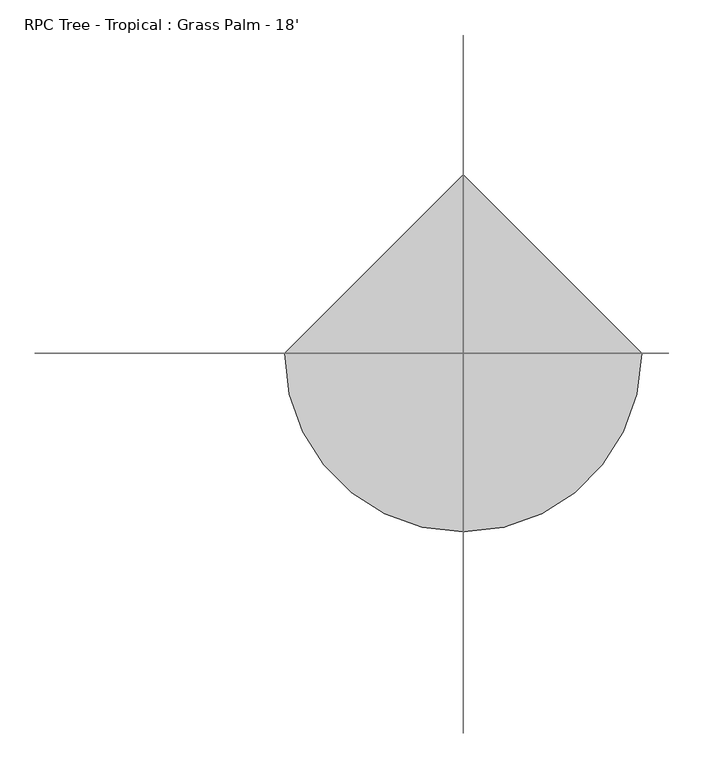
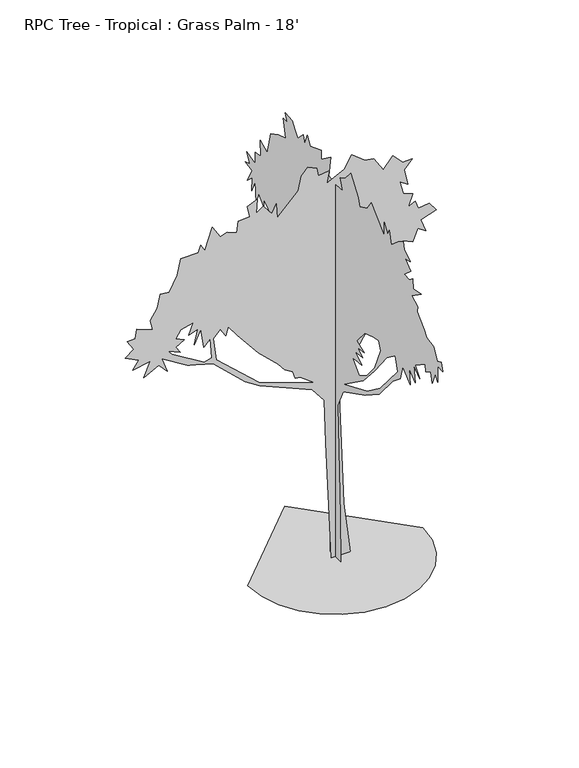
"""IFC4 building model written with IfcOpenShell, lengths in millimetres: geographic element geometry, RPC Tree - Tropical : Grass Palm - 18'."""

from ifc_helpers import new_model, si_unit, origin, place, context, project, spatial, triangles, source, transform, mapped, element, save


def rpc_tree_tropical_grass_palm_18_ffc4a38a(model_context):
    return source(origin(), model_context, "Body", "Tessellation", [
        triangles([(197.8251161, -0.0004657, 0.0001367), (109.1148514, -0.0002635, 694.5605118), (43.5490633, 0.0002048, 2380.5060047), (409.1686295, 0.0003079, 2962.5546341), (570.4154732, 0.000405, 3409.2137077), (607.6747178, 0.0004576, 3623.4372597), (719.4525244, 0.0004509, 3660.6992294), (654.2481468, 0.0004936, 3781.8063721), (747.397621, 0.0005252, 3949.4717194), (775.3401741, 0.0005007, 3874.9480705), (877.80376, 0.0005308, 4042.6134178), (1008.2098989, 0.0004934, 3977.4115837), (1073.4142765, 0.0005291, 4145.0772217), (1175.8753189, 0.0004934, 4070.5535728), (1110.6734848, 0.0005514, 4247.5407349), (1315.5981857, 0.0005381, 4312.742569), (1222.4487843, 0.0005851, 4433.8244225), (1082.7284609, 0.0006012, 4415.2060822), (1039.2334414, 0.0006388, 4529.6586891), (952.3222492, 0.0006386, 4480.4079163), (1008.2098989, 0.0006732, 4638.7514488), (886.9528381, 0.0007051, 4688.7640938), (840.544479, 0.0007593, 4862.3223953), (943.0055214, 0.0007261, 4797.0952721), (896.4321287, 0.0007914, 5011.3441132), (998.8957146, 0.0008063, 5123.1297318), (877.80376, 0.0008246, 5123.1297318), (747.397621, 0.0008797, 5253.5334), (626.3056664, 0.0008575, 5104.4861023), (503.8725509, 0.0009294, 5301.1072403), (384.1216845, 0.0009523, 5318.7352341), (216.4545022, 0.0010156, 5458.4604263), (113.9921609, 0.0009855, 5290.795079), (-109.5623986, 0.0009889, 5179.0094604), (-81.6183375, 0.0010277, 5337.3532837), (-221.3396873, 0.0010437, 5318.7352341), (-239.9693097, 0.0010769, 5430.5202713), (-361.0610281, 0.0011104, 5486.4005814), (-444.8937381, 0.0010978, 5393.2585922), (-482.1529827, 0.0010527, 5206.9496155), (-752.2819885, 0.0010175, 4927.5242294), (-770.9103573, 0.0010735, 5123.1297318), (-826.8005505, 0.0010516, 5011.3441132), (-938.5783207, 0.0011065, 5151.0698868), (-1031.7252514, 0.0011028, 5085.8680527), (-1013.0943392, 0.0011506, 5272.1514496), (-1143.5030216, 0.0011551, 5216.2711395), (-1115.557925, 0.0011104, 5067.2244232), (-1264.5950489, 0.0011304, 5057.9278976), (-1283.2232723, 0.0010926, 4908.8806), (-1404.3152996, 0.0011236, 4955.4643845), (-1497.4622303, 0.0011301, 4927.5242294), (-1599.9257435, 0.0011911, 5095.1895767), (-1702.389402, 0.0011281, 4806.4170868), (-1748.9628674, 0.0011604, 4899.5590759), (-1786.2220757, 0.0011407, 4806.4170868), (-2009.7751453, 0.0011745, 4806.4170868), (-2056.3486107, 0.0011233, 4592.1932442), (-2158.8122692, 0.0010856, 4396.5624527), (-2279.9041512, 0.0011064, 4405.8842674), (-2317.1635048, 0.0010639, 4228.8971054), (-2410.3102901, 0.00104, 4089.1972023), (-2377.0008408, 0.0009991, 3957.4473953), (-2587.2949814, 0.0010515, 4033.2916031), (-2605.9133217, 0.0010214, 3912.2100403), (-2708.3768349, 0.0010343, 3902.8882256), (-2624.5569511, 0.0009862, 3772.4845573), (-2736.3166992, 0.0009803, 3688.6390938), (-2559.355117, 0.0009282, 3595.4973953), (-2633.853186, 0.0009091, 3483.7117767), (-2410.3102901, 0.000888, 3530.2955612), (-2494.1431091, 0.0008475, 3334.6900589), (-2298.535136, 0.0008458, 3437.1535721), (-2186.7573658, 0.000796, 3316.0464294), (-2261.2733116, 0.0008604, 3511.6772209), (-1928.0074619, 0.0007539, 3305.1500015), (-1586.5374619, 0.000677, 3211.8556961), (-1169.4034029, 0.0005069, 2817.7745178), (-980.3029541, 0.0004448, 2694.5084953), (-299.9587802, 0.0002625, 2401.7378483), (-143.374379, 0.000185, 2203.9150394), (-126.1084725, 2.08e-05, 1609.6107628), (-53.6737587, -0.0004278, 0.0001367), (-1497.4622303, 0.0008957, 3651.4027039), (-1422.9462845, 0.000854, 3539.6173759), (-1395.0011879, 0.0008802, 3651.4027039), (-1273.9091606, 0.0008189, 3493.0335915), (-1002.0681953, 0.0003602, 3156.4073364), (-744.7432772, 0.0005791, 2905.2014488), (-659.9860233, 0.000538, 2801.1377426), (-556.6715083, 0.0005054, 2738.5520279), (-519.4122637, 0.0004719, 2636.0885147), (-454.2079225, 0.0004596, 2626.7667), (-267.9141337, 0.0003934, 2487.0438332), (-995.0831566, 0.0005747, 2749.8295372), (-1549.5677708, 0.0007954, 3253.765638), (-1590.6116318, 0.0008844, 3558.2354256), (-2019.0918732, 0.0008854, 3520.9737465), (-2074.9794502, 0.0009166, 3604.8192101), (-1963.20168, 0.0009175, 3670.0207535), (-2074.9794502, 0.0009495, 3725.9007729), (-2009.7751453, 0.0009676, 3828.3645767), (-1851.4239098, 0.0009538, 3865.6262558), (-1907.3141029, 0.0009217, 3716.604538), (-1791.7262455, 0.0009145, 3754.1964294), (-1838.0305412, 0.0008682, 3558.4641907), (-1748.9628674, 0.0009054, 3744.5444023), (-1711.7036591, 0.0008288, 3483.7117767), (-1627.8708401, 0.000839, 3567.5572403), (-1608.65835, 0.0007633, 3299.7651558), (-1708.7927902, 0.0007706, 3271.2916031), (-2130.8671726, 0.0009048, 3530.2955612), (-2177.4431087, 0.000927, 3586.1755806), (0.0001009, -125.9822357, 0.0001592), (6.27e-05, -114.0061317, 632.7801258), (3.21e-05, -52.0852428, 2115.3046051), (1.35e-05, -175.1038104, 2373.6836014), (-6.14e-05, -671.5328476, 2630.4243256), (-0.0001496, -990.5162842, 2836.0117767), (-0.0001562, -1298.9586491, 3200.2479744), (-0.0001816, -1467.3098557, 3334.6900589), (-0.00019, -1523.1974327, 3539.6173759), (-0.0002153, -1690.8629253, 3390.5700783), (-0.0002111, -1662.9202995, 3595.4973953), (-0.0002322, -1802.6406956, 3483.7373566), (-0.0002266, -1765.3814873, 3707.2827232), (-0.0002477, -1905.101738, 3604.8192101), (-0.0002322, -1802.6406956, 3725.9007729), (-0.000266, -2026.196236, 3874.9480705), (-0.0002688, -2044.8246048, 3781.8063721), (-0.0002843, -2147.2882633, 3837.6863914), (-0.0002899, -2184.5450008, 3707.2827232), (-0.0002997, -2249.7493057, 3874.9480705), (-0.0003096, -2314.9536106, 3800.4244217), (-0.0003096, -2314.9536106, 4023.9697884), (-0.0003265, -2426.7289101, 4014.6735535), (-0.0003208, -2389.4721725, 4126.4335922), (-0.0003068, -2296.3227711, 4079.8753876), (-0.0002955, -2221.8042091, 4238.2189201), (-0.0002716, -2063.4555897, 4266.1590752), (-0.0002632, -2007.5653965, 4340.6824333), (-0.0002792, -1849.2141609, 4489.729731), (-0.0002806, -1858.5282726, 4564.2280907), (-0.0002609, -1728.1221336, 4638.7514488), (-0.0002933, -1942.3609463, 4787.7987465), (-0.0002652, -1756.0672302, 4750.5370674), (-0.0002638, -1746.7531185, 4880.9404449), (-0.0002525, -1672.2345566, 4825.0607162), (-0.0002356, -1560.4567863, 4834.3569511), (-0.0002567, -1700.177037, 4955.4643845), (-0.0002384, -1579.0876259, 5057.9278976), (-0.0002553, -1690.8629253, 5085.8680527), (-0.0002342, -1551.1425293, 5169.6879364), (-0.0002314, -1532.5116898, 5262.854924), (-0.0002145, -1420.7339195, 5197.6530899), (-0.0001906, -1262.3826839, 5057.9278976), (-0.0001836, -1215.8092186, 5225.5932449), (-0.000178, -1178.5499376, 5151.0698868), (-0.0002067, -1104.0339191, 5272.1514496), (-0.0001667, -1104.0339191, 5085.8680527), (-0.0001811, -934.8191025, 5242.9666031), (-0.0001617, -805.9598167, 5355.9969131), (-0.0001497, -726.4933737, 5236.9472031), (-0.0001237, -554.4617231, 5151.0698868), (-0.0001181, -517.2024785, 5253.5334), (-9.28e-05, -349.5370585, 5486.4005814), (-7.45e-05, -228.4440684, 5346.6748077), (-5.62e-05, -107.3520956, 5281.4729736), (-6.46e-05, -163.2409807, 5132.4512558), (-4.21e-05, -14.2045188, 5123.1297318), (-1.82e-05, 144.1465339, 5151.0698868), (-2.38e-05, 106.8877798, 5430.5202713), (7.1e-06, 311.8129804, 5281.4729736), (7.1e-06, 311.8129804, 5402.5551178), (4.51e-05, 563.311074, 5309.4131287), (5.49e-05, 628.5154152, 5421.1987473), (6.48e-05, 693.7172493, 5262.854924), (6.9e-05, 721.6623459, 5365.3184372), (8.73e-05, 842.7543005, 5244.2112946), (9.71e-05, 907.9586054, 5309.4131287), (0.000107, 973.1604395, 5411.8766418), (9.09e-05, 1131.5116751, 5421.1987473), (0.0001238, 1084.9382097, 5318.7352341), (0.0001369, 1171.5319067, 5326.1010635), (0.0001281, 1112.8833063, 5085.8680527), (0.0001548, 1289.862838, 5020.6662186), (0.0001793, 1452.3822784, 4938.471817), (0.0001914, 1532.0468925, 4629.4296341), (0.0002153, 1690.3981281, 4703.9532829), (0.0002139, 1681.0838711, 4489.729731), (0.0002321, 1802.1758984, 4471.0861015), (0.0002321, 1802.1758984, 4312.742569), (0.0002617, 1997.7863422, 4359.3007736), (0.0002506, 1924.1873463, 4240.2763527), (0.0002671, 2033.8797787, 4204.1576271), (0.0002434, 1876.6944603, 4173.017086), (0.0002603, 1988.4722305, 3977.4115837), (0.000242, 1867.3802032, 4079.8753876), (0.0002448, 1886.008572, 3893.5664108), (0.0002321, 1802.1758984, 4070.5535728), (0.0002293, 1783.5475296, 3791.102607), (0.0002209, 1727.6573364, 3949.4717194), (0.000204, 1615.8795662, 3837.6863914), (0.000204, 1615.8795662, 3940.1499046), (0.0001974, 1307.620039, 3736.3911209), (0.0001385, 917.2727898, 3623.4372597), (0.0001194, 790.5928768, 3229.1531868), (0.0001184, 784.0523603, 3133.6235527), (0.0001019, 675.0888805, 3064.5609077), (0.0001273, 842.7543005, 2934.1575302), (0.0001104, 730.9765303, 2971.4192093), (0.0001532, 749.6048264, 2775.813707), (0.0001377, 647.143784, 2906.2173752), (0.0001349, 628.5154152, 2673.3501938), (0.0001307, 600.5703549, 2775.813707), (0.0001264, 572.6252584, 2673.3501938), (0.0001194, 526.0518293, 2841.0155411), (0.0001152, 498.1067327, 2682.6467194), (0.0001124, 479.478364, 2608.1483597), (0.0001067, 442.2191194, 2738.5520279), (9.69e-05, 377.0147781, 2654.7065643), (7.78e-05, 250.6550855, 2492.941729), (2.45e-05, 161.9890223, 2108.946999), (9.68e-05, 111.8545007, 1061.9156324), (0.0001375, 116.2017099, 0.0001159), (-9.51e-05, -630.0470804, 2801.0107155), (-0.0001338, -885.9978092, 3096.8699821), (-0.0001753, -1160.7521868, 3441.0905411), (-0.0002047, -1355.5320854, 3586.1755806), (-0.0002131, -1411.4196625, 3399.891893), (-0.0001538, -1018.750898, 2931.8969124), (-0.0001089, -721.0450871, 2712.8219124), (-2.89e-05, -191.1855686, 2487.0438332), (-6.83e-05, -451.9981009, 2980.7157349), (-8.93e-05, -591.7210041, 2990.0375496), (-6.83e-05, -451.9981009, 3092.5010628), (-9.36e-05, -619.6661007, 3111.1446922), (-7.67e-05, -507.7485861, 3183.8393829), (-9.92e-05, -656.9227655, 3204.2863907), (-7.39e-05, -489.2573819, 3269.4882248), (-0.0001003, -664.5148893, 3478.2763527), (-0.0001315, -871.1641943, 3548.9391907), (-0.0001484, -982.9419645, 3567.5572403), (-0.0001546, -1023.6937649, 3456.6608116), (-0.0001342, -889.0838854, 3136.1382248), (-0.0001091, -722.497978, 2934.7415062), (-8.09e-05, -535.8308109, 2813.0500969), (-5.98e-05, -396.1104876, 2971.4192093), (-1140.1273556, 0.0, 0.0001367), (-1109.9876982, -261.2415577, 0.0001834), (-1024.1458448, -501.1521864, 0.0002263), (-889.4750679, -712.8535812, 0.0002641), (-712.8535812, -889.4750679, 0.0002957), (-501.1496429, -1024.1458448, 0.0), (-261.2415577, -1109.9876982, 1.53e-05), (6.77e-05, -1140.1273556, 2.07e-05), (261.2415577, -1109.9876982, 1.53e-05), (501.1521864, -1024.1458448, 0.0), (712.8535812, -889.4750679, 0.0002957), (889.4750679, -712.8535812, 0.0002641), (1024.1458448, -501.1496429, 0.0002263), (1109.9876982, -261.2415577, 0.0001834), (1140.1273556, 9.97e-05, 0.0001367), (-0.0001476, 1140.1273556, 0.0002526)], [[95, 110, 96], [86, 3, 87], [87, 3, 88], [88, 3, 89], [106, 105, 107], [89, 3, 90], [90, 3, 91], [74, 73, 75], [42, 41, 43], [14, 13, 15], [98, 113, 99], [72, 71, 73], [96, 110, 97], [110, 109, 97], [70, 69, 71], [24, 23, 25], [26, 25, 27], [85, 84, 86], [55, 54, 56], [53, 52, 54], [104, 103, 105], [10, 9, 11], [108, 107, 109], [100, 99, 101], [46, 45, 47], [47, 45, 48], [66, 65, 67], [68, 67, 69], [16, 15, 17], [17, 15, 18], [35, 34, 36], [73, 71, 75], [64, 63, 65], [7, 6, 8], [3, 86, 4], [19, 18, 20], [32, 31, 33], [1, 83, 2], [83, 82, 2], [2, 82, 3], [82, 81, 3], [28, 27, 29], [12, 11, 13], [81, 80, 3], [4, 86, 5], [5, 86, 6], [21, 20, 22], [44, 43, 45], [27, 25, 29], [25, 23, 29], [60, 59, 61], [99, 113, 101], [49, 48, 50], [57, 56, 58], [6, 86, 8], [38, 37, 39], [37, 36, 39], [39, 36, 40], [36, 34, 40], [65, 63, 67], [67, 63, 69], [69, 63, 71], [71, 63, 75], [92, 91, 93], [91, 3, 93], [93, 3, 94], [3, 80, 94], [80, 79, 94], [94, 79, 95], [79, 78, 95], [95, 78, 110], [78, 77, 110], [110, 77, 111], [77, 76, 111], [111, 76, 112], [76, 75, 112], [112, 75, 113], [75, 63, 113], [113, 63, 101], [101, 63, 102], [97, 109, 84], [109, 107, 84], [8, 86, 9], [63, 62, 102], [62, 61, 102], [61, 59, 102], [102, 59, 103], [59, 58, 103], [58, 56, 103], [56, 54, 103], [18, 15, 20], [15, 13, 20], [13, 11, 20], [54, 52, 103], [52, 51, 103], [51, 50, 103], [103, 50, 105], [105, 50, 107], [107, 50, 84], [84, 50, 86], [86, 50, 9], [50, 48, 9], [48, 45, 9], [40, 34, 41], [30, 29, 31], [31, 29, 33], [33, 29, 34], [11, 9, 20], [29, 23, 34], [23, 22, 34], [34, 22, 41], [22, 20, 41], [20, 9, 41], [9, 45, 41], [45, 43, 41], [226, 245, 246], [245, 226, 227], [233, 116, 117], [126, 127, 128], [209, 210, 211], [198, 199, 200], [213, 214, 215], [196, 197, 198], [226, 246, 247], [200, 201, 202], [144, 145, 146], [238, 239, 240], [194, 195, 196], [218, 219, 220], [215, 216, 217], [158, 159, 160], [211, 212, 213], [245, 227, 228], [244, 245, 228], [131, 132, 133], [236, 237, 238], [234, 235, 236], [122, 123, 124], [133, 134, 135], [124, 125, 126], [156, 157, 158], [233, 226, 247], [192, 193, 194], [202, 203, 204], [151, 152, 153], [171, 172, 173], [175, 176, 177], [233, 117, 118], [232, 233, 118], [232, 118, 119], [231, 232, 119], [231, 119, 120], [230, 231, 120], [230, 120, 121], [217, 218, 220], [230, 121, 122], [229, 230, 122], [146, 147, 148], [177, 178, 179], [181, 182, 183], [188, 189, 190], [135, 136, 137], [135, 137, 138], [213, 215, 217], [173, 174, 175], [153, 154, 155], [183, 184, 185], [129, 130, 131], [165, 166, 167], [149, 150, 151], [161, 162, 163], [180, 181, 183], [192, 194, 196], [225, 114, 115], [224, 225, 115], [224, 115, 116], [223, 224, 116], [156, 158, 160], [233, 247, 248], [180, 183, 185], [179, 180, 185], [209, 211, 213], [167, 168, 169], [165, 167, 169], [164, 165, 169], [190, 191, 192], [248, 234, 236], [222, 223, 116], [222, 116, 233], [196, 198, 200], [222, 233, 248], [221, 222, 248], [220, 221, 248], [142, 143, 144], [217, 220, 248], [192, 196, 200], [151, 153, 155], [151, 155, 156], [149, 151, 156], [243, 244, 228], [243, 228, 229], [144, 146, 148], [144, 148, 149], [217, 248, 236], [138, 139, 140], [207, 208, 209], [200, 202, 204], [192, 200, 204], [190, 192, 204], [188, 190, 204], [188, 204, 205], [188, 205, 206], [209, 213, 217], [209, 217, 236], [209, 236, 238], [209, 238, 240], [207, 209, 240], [206, 207, 240], [206, 240, 241], [188, 206, 241], [187, 188, 241], [186, 187, 241], [185, 186, 241], [179, 185, 241], [177, 179, 241], [175, 177, 241], [173, 175, 241], [171, 173, 241], [170, 171, 241], [169, 170, 241], [164, 169, 241], [164, 241, 242], [164, 242, 243], [163, 164, 243], [161, 163, 243], [160, 161, 243], [160, 243, 229], [156, 160, 229], [149, 156, 229], [144, 149, 229], [142, 144, 229], [141, 142, 229], [141, 229, 122], [141, 122, 124], [141, 124, 126], [141, 126, 128], [141, 128, 129], [140, 141, 129], [138, 140, 129], [138, 129, 131], [138, 131, 133], [138, 133, 135], [263, 264, 249], [262, 263, 249], [262, 249, 250], [261, 262, 250], [261, 250, 251], [261, 251, 252], [260, 261, 252], [259, 260, 252], [259, 252, 253], [259, 253, 254], [259, 254, 255], [259, 255, 256], [259, 256, 257], [259, 257, 258]], closed=False),
    ])


if __name__ == "__main__":
    model = new_model("IFC4")
    model_context = context("Model", 3, world=origin())
    ifc_project = project(units=[si_unit("LENGTHUNIT", "METRE", prefix="MILLI")], contexts=[model_context])
    site = spatial("IfcSite", under=ifc_project)
    building = spatial("IfcBuilding", under=site)
    placement = place(None, origin())
    rpc_tree_tropical_grass_palm_18_shape = rpc_tree_tropical_grass_palm_18_ffc4a38a(model_context)
    element("IfcGeographicElement", 1, ObjectType="RPC Tree - Tropical : Grass Palm - 18'", at=placement, inside=building, context=model_context, shape_type="MappedRepresentation", body=[
        mapped(rpc_tree_tropical_grass_palm_18_shape, transform((0.0, 0.0, 0.0), x_axis=(1.0, 0.0, 0.0), y_axis=(0.0, 1.0, 0.0), z_axis=(0.0, 0.0, 1.0))),
    ])
    save(model, "model.ifc")

# Revit data of these elements
# Type "RPC Tree - Tropical : Grass Palm - 18'"
#   built-in parameter 1005198 = "{2, 15},{39, RPC-16-FXGK-2WG0-PNFG-U000-ST1L-LVER-AU},{1, 0},{1, 0},{2, 35},{1, 8},{5, Color},{1, 0},{1, 0},{3, 0.8},{3, 0.8},{3, 0.8},{1, 8},{7, BBoxMin},{1, 0},{1, 0},{1, 0},{1, 0},{1, 0},{1, 8},{7, BBoxMax},{1, 0},{1, 0},{1, 0},{1, 0},{1, 0},{2, 11},{9, RPCTypeId},{1, 0},{1, 0},{39, RPC-16-FXGK-2WG0-PNFG-U000-ST1L-LVER-AU},{1, 6},{14, RPCPlantHeight},{1, 0},{1, 0},{2, 18},{2, 11},{7, keyword},{1, 0},{1, 0},{76, :Geometry:RPC:Grass Palm:cordyline australis:grass palm:tropical:trees:beach},{2, 11},{8, category},{1, 0},{1, 0},{17, :Trees [Tropical]},{2, 11},{12, LocalizedUID},{1, 0},{1, 0},{10, Grass Palm},{2, 14},{6, Height},{1, 0},{1, 0},{2, 18},{1, 2},{16, Cast Reflections},{1, 0},{1, 0},{1, 0},{1, 2},{12, Cast Shadows},{1, 0},{1, 0},{1, 1},{1, 2},{9, Lock View},{1, 0},{1, 0},{1, 0},{1, 4},{5, ViewC},{1, 0},{1, 0},{1, 0},{2, 11},{20, AdvancedUIDefinition},{1, 0},{1, 0},{0, },{2, 11},{10, AssetLibID},{1, 0},{1, 0},{36, 4D3F6E72-3F99-4203-98E9-AF80B3C7A7A4},{2, 11},{10, BaseSchema},{1, 0},{1, 0},{9, RPCSchema},{2, 11},{12, ExchangeGUID},{1, 0},{1, 0},{0, },{1, 2},{6, Hidden},{1, 0},{1, 0},{1, 0},{1, 4},{11, RPCCategory},{1, 0},{1, 0},{1, 0},{2, 11},{8, RPCImage},{1, 0},{1, 0},{0, },{1, 4},{13, SchemaVersion},{1, 0},{1, 0},{1, 4},{2, 11},{12, UIDefinition},{1, 0},{1, 0},{0, },{2, 11},{6, UIName},{1, 0},{1, 0},{39, RPC-16-FXGK-2WG0-PNFG-U000-ST1L-LVER-AU},{2, 11},{11, VersionGUID},{1, 0},{1, 0},{9, RPCSchema},{2, 11},{9, assettype},{1, 0},{1, 0},{11, RPCGeometry},{2, 11},{11, description},{1, 0},{1, 0},{0, },{2, 11},{9, localname},{1, 0},{1, 0},{3, RPC},{2, 11},{9, localtype},{1, 0},{1, 0},{3, RPC},{1, 4},{8, revision},{1, 0},{1, 0},{1, 1},{2, 11},{9, thumbnail},{1, 0},{1, 0},{0, },{1, 4},{7, version},{1, 0},{1, 0},{1, 1},{1, 2},{20, RPC_Cast Reflections},{1, 0},{1, 0},{1, 1},{1, 2},{16, RPC_Cast Shadows},{1, 0},{1, 0},{1, 1},{1, 2},{13, RPC_Lock View},{1, 0},{1, 0},{1, 0},{1, 4},{9, RPC_ViewC},{1, 0},{1, 0},{1, 0},{21, assetlibrary_base.fbx},{1, 5},"
#   built-in parameter 1005195 = "RPC-16-FXGK-2WG0-PNFG-U000-ST1L-LVER-AU"
#   Type Comments = "Grass Palm"
#   Assembly Code = "G2050500"
#   Height = 18' - 0"
#   Plan Symbol = element 419189
#   Default Elevation = 0
